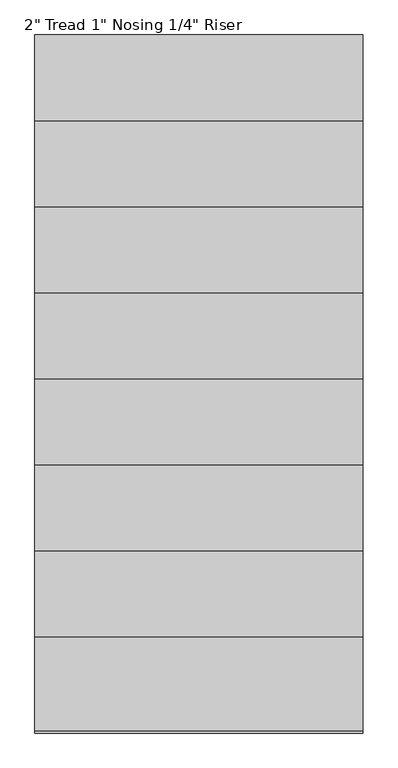
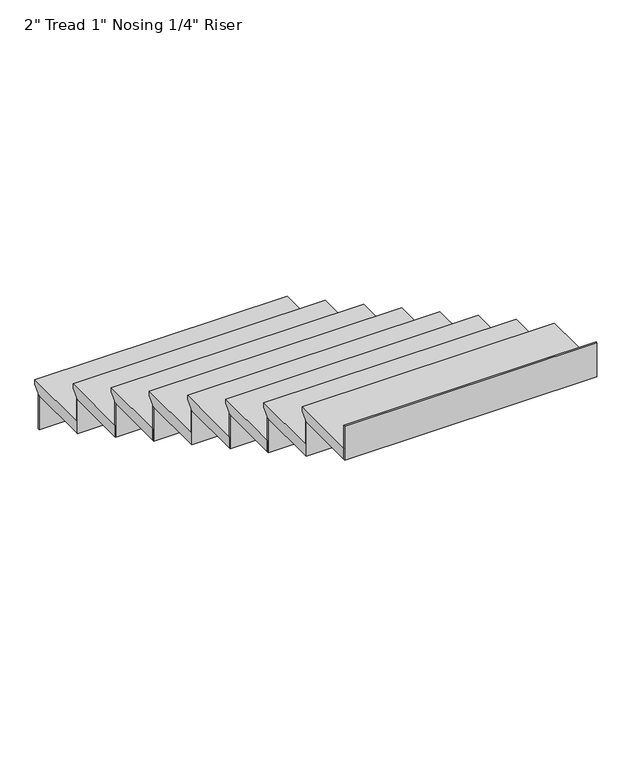
"""IFC4 building model written with IfcOpenShell, lengths in millimetres: stair flight geometry."""

from ifc_helpers import new_model, si_unit, frame, origin, place, context, project, spatial, polyline, outline, extrude, source, transform, mapped, element, save


def stair_flight_a6ac55d9(model_context):
    return source(origin(), model_context, "Body", "SweptSolid", [
        extrude(outline(polyline([(-2204.7834702, 7924.8), (-1899.9834702, 7924.8), (-1899.9834702, 7905.75), (-1925.3834702, 7880.35), (-1925.3834702, 7874.0), (-2204.7834702, 7874.0), (-2204.7834702, 7924.8)])), frame((2385.53354, 0.0, 0.0), z_axis=(1.0, 0.0, 0.0), x_axis=(0.0, 1.0, 0.0)), (0.0, 0.0, 1.0), 1066.8),
        extrude(outline(polyline([(2385.53354, -1931.7334702), (2385.53354, -1925.3834702), (3452.33354, -1925.3834702), (3452.33354, -1931.7334702), (2385.53354, -1931.7334702)])), frame((0.0, 0.0, 7721.6), z_axis=(0.0, 0.0, 1.0), x_axis=(1.0, 0.0, 0.0)), (0.0, 0.0, 1.0), 152.4),
        extrude(outline(polyline([(2385.53354, -2211.1334702), (2385.53354, -2204.7834702), (3452.33354, -2204.7834702), (3452.33354, -2211.1334702), (2385.53354, -2211.1334702)])), frame((0.0, 0.0, 7874.0), z_axis=(0.0, 0.0, 1.0), x_axis=(1.0, 0.0, 0.0)), (0.0, 0.0, 1.0), 152.4),
        extrude(outline(polyline([(-2484.1834702, 8077.2), (-2179.3834702, 8077.2), (-2179.3834702, 8058.15), (-2204.7834702, 8032.75), (-2204.7834702, 8026.4), (-2484.1834702, 8026.4), (-2484.1834702, 8077.2)])), frame((2385.53354, 0.0, 0.0), z_axis=(1.0, 0.0, 0.0), x_axis=(0.0, 1.0, 0.0)), (0.0, 0.0, 1.0), 1066.8),
        extrude(outline(polyline([(2385.53354, -2490.5334702), (2385.53354, -2484.1834702), (3452.33354, -2484.1834702), (3452.33354, -2490.5334702), (2385.53354, -2490.5334702)])), frame((0.0, 0.0, 8026.4), z_axis=(0.0, 0.0, 1.0), x_axis=(1.0, 0.0, 0.0)), (0.0, 0.0, 1.0), 152.4),
        extrude(outline(polyline([(-2763.5834702, 8229.6), (-2458.7834702, 8229.6), (-2458.7834702, 8210.55), (-2484.1834702, 8185.15), (-2484.1834702, 8178.8), (-2763.5834702, 8178.8), (-2763.5834702, 8229.6)])), frame((2385.53354, 0.0, 0.0), z_axis=(1.0, 0.0, 0.0), x_axis=(0.0, 1.0, 0.0)), (0.0, 0.0, 1.0), 1066.8),
        extrude(outline(polyline([(2385.53354, -2769.9334702), (2385.53354, -2763.5834702), (3452.33354, -2763.5834702), (3452.33354, -2769.9334702), (2385.53354, -2769.9334702)])), frame((0.0, 0.0, 8178.8), z_axis=(0.0, 0.0, 1.0), x_axis=(1.0, 0.0, 0.0)), (0.0, 0.0, 1.0), 152.4),
        extrude(outline(polyline([(-3042.9834702, 8382.0), (-2738.1834702, 8382.0), (-2738.1834702, 8362.95), (-2763.5834702, 8337.55), (-2763.5834702, 8331.2), (-3042.9834702, 8331.2), (-3042.9834702, 8382.0)])), frame((2385.53354, 0.0, 0.0), z_axis=(1.0, 0.0, 0.0), x_axis=(0.0, 1.0, 0.0)), (0.0, 0.0, 1.0), 1066.8),
        extrude(outline(polyline([(2385.53354, -3049.3334702), (2385.53354, -3042.9834702), (3452.33354, -3042.9834702), (3452.33354, -3049.3334702), (2385.53354, -3049.3334702)])), frame((0.0, 0.0, 8331.2), z_axis=(0.0, 0.0, 1.0), x_axis=(1.0, 0.0, 0.0)), (0.0, 0.0, 1.0), 152.4),
        extrude(outline(polyline([(-3322.3834702, 8534.4), (-3017.5834702, 8534.4), (-3017.5834702, 8515.35), (-3042.9834702, 8489.95), (-3042.9834702, 8483.6), (-3322.3834702, 8483.6), (-3322.3834702, 8534.4)])), frame((2385.53354, 0.0, 0.0), z_axis=(1.0, 0.0, 0.0), x_axis=(0.0, 1.0, 0.0)), (0.0, 0.0, 1.0), 1066.8),
        extrude(outline(polyline([(2385.53354, -3328.7334702), (2385.53354, -3322.3834702), (3452.33354, -3322.3834702), (3452.33354, -3328.7334702), (2385.53354, -3328.7334702)])), frame((0.0, 0.0, 8483.6), z_axis=(0.0, 0.0, 1.0), x_axis=(1.0, 0.0, 0.0)), (0.0, 0.0, 1.0), 152.4),
        extrude(outline(polyline([(-3601.7834702, 8686.8), (-3296.9834702, 8686.8), (-3296.9834702, 8667.75), (-3322.3834702, 8642.35), (-3322.3834702, 8636.0), (-3601.7834702, 8636.0), (-3601.7834702, 8686.8)])), frame((2385.53354, 0.0, 0.0), z_axis=(1.0, 0.0, 0.0), x_axis=(0.0, 1.0, 0.0)), (0.0, 0.0, 1.0), 1066.8),
        extrude(outline(polyline([(2385.53354, -3608.1334702), (2385.53354, -3601.7834702), (3452.33354, -3601.7834702), (3452.33354, -3608.1334702), (2385.53354, -3608.1334702)])), frame((0.0, 0.0, 8636.0), z_axis=(0.0, 0.0, 1.0), x_axis=(1.0, 0.0, 0.0)), (0.0, 0.0, 1.0), 152.4),
        extrude(outline(polyline([(-3881.1834702, 8839.2), (-3576.3834702, 8839.2), (-3576.3834702, 8820.15), (-3601.7834702, 8794.75), (-3601.7834702, 8788.4), (-3881.1834702, 8788.4), (-3881.1834702, 8839.2)])), frame((2385.53354, 0.0, 0.0), z_axis=(1.0, 0.0, 0.0), x_axis=(0.0, 1.0, 0.0)), (0.0, 0.0, 1.0), 1066.8),
        extrude(outline(polyline([(2385.53354, -3887.5334702), (2385.53354, -3881.1834702), (3452.33354, -3881.1834702), (3452.33354, -3887.5334702), (2385.53354, -3887.5334702)])), frame((0.0, 0.0, 8788.4), z_axis=(0.0, 0.0, 1.0), x_axis=(1.0, 0.0, 0.0)), (0.0, 0.0, 1.0), 152.4),
        extrude(outline(polyline([(2385.53354, -4166.9334702), (2385.53354, -4160.5834702), (3452.33354, -4160.5834702), (3452.33354, -4166.9334702), (2385.53354, -4166.9334702)])), frame((0.0, 0.0, 8940.8), z_axis=(0.0, 0.0, 1.0), x_axis=(1.0, 0.0, 0.0)), (0.0, 0.0, 1.0), 152.4),
        extrude(outline(polyline([(-4160.5834702, 8991.6), (-3855.7834702, 8991.6), (-3855.7834702, 8972.55), (-3881.1834702, 8947.15), (-3881.1834702, 8940.8), (-4160.5834702, 8940.8), (-4160.5834702, 8991.6)])), frame((2385.53354, 0.0, 0.0), z_axis=(1.0, 0.0, 0.0), x_axis=(0.0, 1.0, 0.0)), (0.0, 0.0, 1.0), 1066.8),
    ])


if __name__ == "__main__":
    model = new_model("IFC4")
    model_context = context("Model", 3, world=origin())
    ifc_project = project(units=[si_unit("LENGTHUNIT", "METRE", prefix="MILLI")], contexts=[model_context])
    site = spatial("IfcSite", under=ifc_project)
    building = spatial("IfcBuilding", under=site)
    placement = place(None, origin())
    stair_flight_shape = stair_flight_a6ac55d9(model_context)
    element("IfcStairFlight", 1, ObjectType="2\" Tread 1\" Nosing 1/4\" Riser", at=placement, inside=building, context=model_context, shape_type="MappedRepresentation", body=[
        mapped(stair_flight_shape, transform((0.0, 0.0, 0.0), x_axis=(1.0, 0.0, 0.0), y_axis=(0.0, 1.0, 0.0), z_axis=(0.0, 0.0, 1.0))),
    ])
    save(model, "model.ifc")
